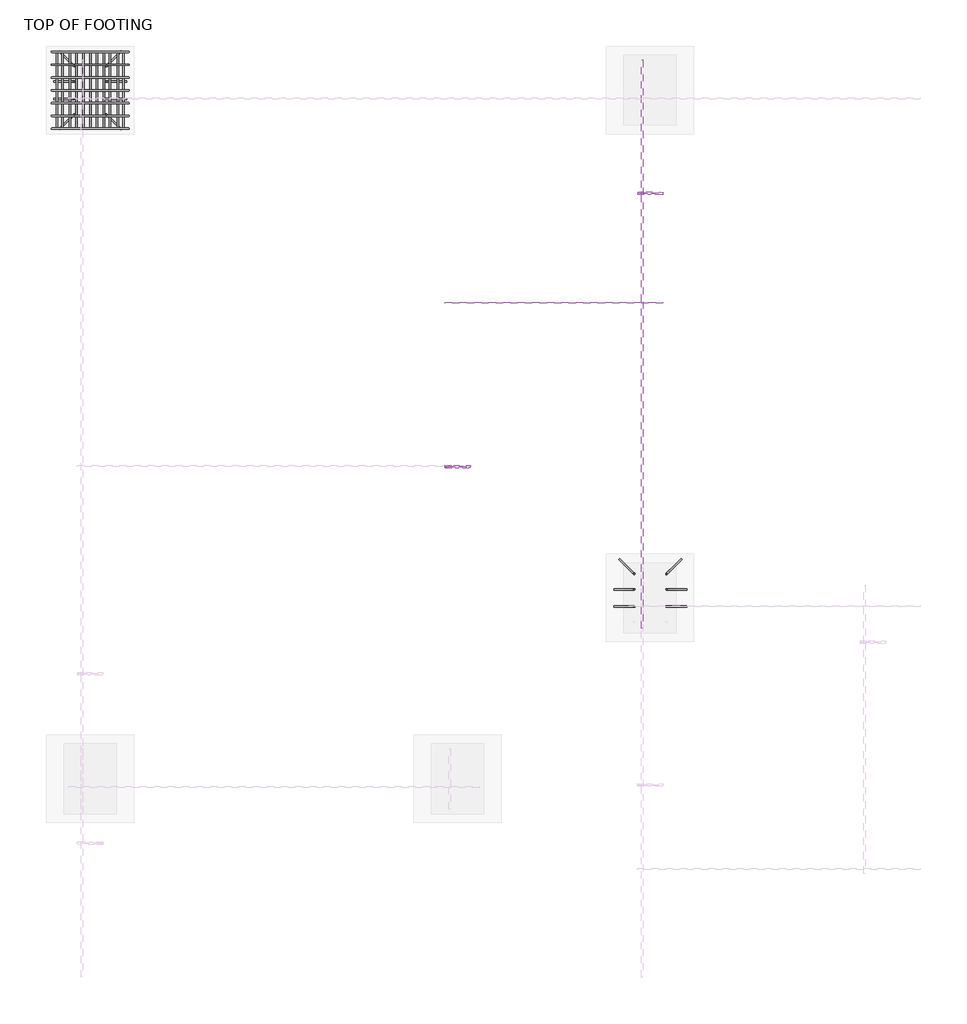
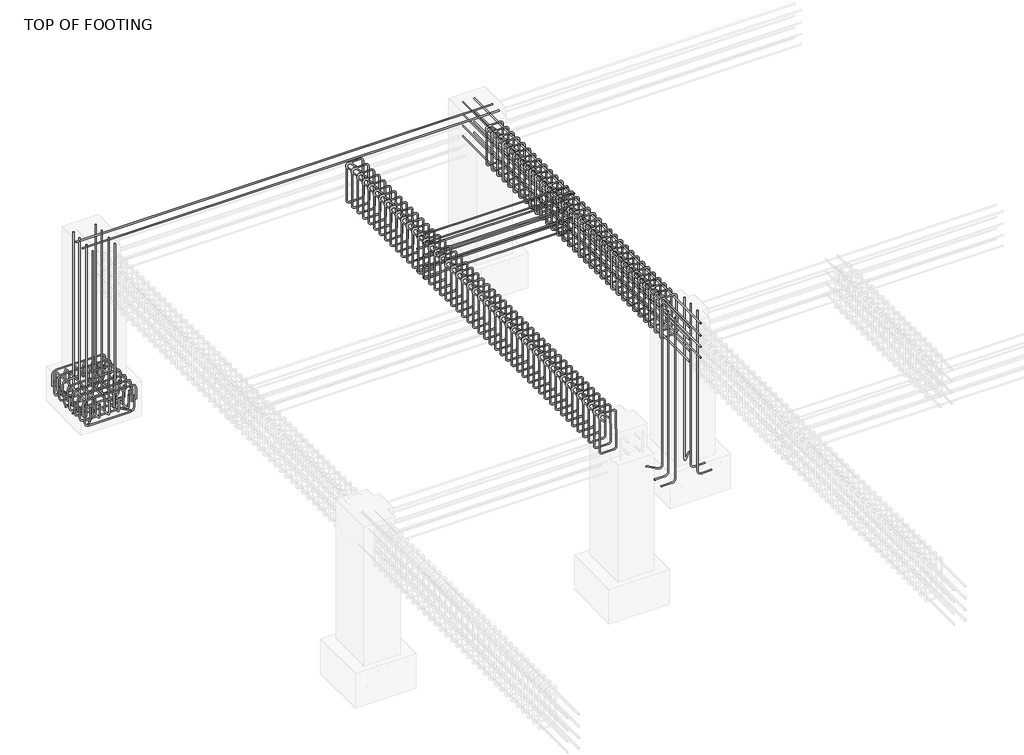
# One storey, part 6 of 8: 25 reinforcing bars.
"""IFC4 building model written with IfcOpenShell, lengths in millimetres."""

from ifc_helpers import new_model, si_unit, point, frame, origin, place, context, project, spatial, polyline, circle_curve, trimmed, segment, composite_curve, source, transform, mapped, element, save
from ifc_brep_helpers import swept_disk

model = new_model("IFC4")

# Units and contexts
model_context = context("Model", 3, world=origin())
ifc_project = project(units=[si_unit("LENGTHUNIT", "METRE", prefix="MILLI")], contexts=[model_context])

# Site, building, storey
site = spatial("IfcSite", under=ifc_project)
building = spatial("IfcBuilding", under=site)
storey = spatial("IfcBuildingStorey", under=building, Name="TOP OF FOOTING", Elevation=-1828.8)

# Reinforcing bars
placement = place(None, origin())
reinforcing_bar_shape = source(origin(), model_context, "Body", "SolidModel", [
    swept_disk(composite_curve([segment(polyline([(-6195.5877818, 9895.6420243, -2021.245224), (-6195.5877818, 9895.6420243, -2168.545224)]), True, "CONTINUOUS"), segment(trimmed(circle_curve(frame((-6241.9377818, 9895.6420243, -2168.545224), z_axis=(0.0, 1.0, 0.0), x_axis=(46.350000000000364, 0.0, 0.0)), 46.35), [point((-6195.5877818, 9895.6420243, -2168.545224))], [point((-6241.9377818, 9895.6420243, -2214.895224))], True, "CARTESIAN"), True, "CONTINUOUS"), segment(polyline([(-6241.9377818, 9895.6420243, -2214.895224), (-6762.8758647, 9895.6420243, -2214.895224)]), True, "CONTINUOUS"), segment(trimmed(circle_curve(frame((-6762.8758647, 9895.6420243, -2168.545224), z_axis=(0.0, 1.0, 0.0), x_axis=(0.0, 0.0, -46.34999999999991)), 46.35), [point((-6762.8758647, 9895.6420243, -2214.895224))], [point((-6809.2258647, 9895.6420243, -2168.545224))], True, "CARTESIAN"), True, "CONTINUOUS"), segment(polyline([(-6809.2258647, 9895.6420243, -2168.545224), (-6809.2258647, 9895.6420243, -2021.245224)]), True, "CONTINUOUS")], self_intersect=False), 6.35),
])
element("IfcReinforcingBar", 1, at=placement, inside=storey, context=model_context, shape_type="MappedRepresentation", body=[
    mapped(reinforcing_bar_shape, transform((0.0, 0.0, 0.0), x_axis=(1.0, 0.0, 0.0), y_axis=(0.0, 1.0, 0.0), z_axis=(0.0, 0.0, 1.0))),
    mapped(reinforcing_bar_shape, transform((0.0, -109.55, 0.0), x_axis=(1.0, 0.0, 0.0), y_axis=(0.0, 1.0, 0.0), z_axis=(0.0, 0.0, 1.0))),
    mapped(reinforcing_bar_shape, transform((0.0, -219.1, 0.0), x_axis=(1.0, 0.0, 0.0), y_axis=(0.0, 1.0, 0.0), z_axis=(0.0, 0.0, 1.0))),
    mapped(reinforcing_bar_shape, transform((0.0, -328.65, 0.0), x_axis=(1.0, 0.0, 0.0), y_axis=(0.0, 1.0, 0.0), z_axis=(0.0, 0.0, 1.0))),
    mapped(reinforcing_bar_shape, transform((0.0, -438.2, 0.0), x_axis=(1.0, 0.0, 0.0), y_axis=(0.0, 1.0, 0.0), z_axis=(0.0, 0.0, 1.0))),
    mapped(reinforcing_bar_shape, transform((0.0, -547.75, 0.0), x_axis=(1.0, 0.0, 0.0), y_axis=(0.0, 1.0, 0.0), z_axis=(0.0, 0.0, 1.0))),
    mapped(reinforcing_bar_shape, transform((0.0, -657.3, 0.0), x_axis=(1.0, 0.0, 0.0), y_axis=(0.0, 1.0, 0.0), z_axis=(0.0, 0.0, 1.0))),
])
reinforcing_bar_2_shape = source(origin(), model_context, "Body", "SolidModel", [
    swept_disk(composite_curve([segment(polyline([(-6831.1461367, 9895.6420243, -2068.8), (-6831.1461367, 9895.6420243, -1921.5)]), True, "CONTINUOUS"), segment(trimmed(circle_curve(frame((-6784.7961367, 9895.6420243, -1921.5), z_axis=(0.0, 1.0, 0.0), x_axis=(-46.350000000000364, 0.0, 0.0)), 46.35), [point((-6831.1461367, 9895.6420243, -1921.5))], [point((-6784.7961367, 9895.6420243, -1875.15))], True, "CARTESIAN"), True, "CONTINUOUS"), segment(polyline([(-6784.7961367, 9895.6420243, -1875.15), (-6220.1961367, 9895.6420243, -1875.15)]), True, "CONTINUOUS"), segment(trimmed(circle_curve(frame((-6220.1961367, 9895.6420243, -1921.5), z_axis=(0.0, 1.0, 0.0), x_axis=(0.0, 0.0, 46.34999999999991)), 46.35), [point((-6220.1961367, 9895.6420243, -1875.15))], [point((-6173.8461367, 9895.6420243, -1921.5))], True, "CARTESIAN"), True, "CONTINUOUS"), segment(polyline([(-6173.8461367, 9895.6420243, -1921.5), (-6173.8461367, 9895.6420243, -2068.8)]), True, "CONTINUOUS")], self_intersect=False), 6.35),
])
element("IfcReinforcingBar", 2, at=placement, inside=storey, context=model_context, shape_type="MappedRepresentation", body=[
    mapped(reinforcing_bar_2_shape, transform((0.0, 0.0, 0.0), x_axis=(1.0, 0.0, 0.0), y_axis=(0.0, 1.0, 0.0), z_axis=(0.0, 0.0, 1.0))),
    mapped(reinforcing_bar_2_shape, transform((0.0, -109.55, 0.0), x_axis=(1.0, 0.0, 0.0), y_axis=(0.0, 1.0, 0.0), z_axis=(0.0, 0.0, 1.0))),
    mapped(reinforcing_bar_2_shape, transform((0.0, -219.1, 0.0), x_axis=(1.0, 0.0, 0.0), y_axis=(0.0, 1.0, 0.0), z_axis=(0.0, 0.0, 1.0))),
    mapped(reinforcing_bar_2_shape, transform((0.0, -328.65, 0.0), x_axis=(1.0, 0.0, 0.0), y_axis=(0.0, 1.0, 0.0), z_axis=(0.0, 0.0, 1.0))),
    mapped(reinforcing_bar_2_shape, transform((0.0, -438.2, 0.0), x_axis=(1.0, 0.0, 0.0), y_axis=(0.0, 1.0, 0.0), z_axis=(0.0, 0.0, 1.0))),
    mapped(reinforcing_bar_2_shape, transform((0.0, -547.75, 0.0), x_axis=(1.0, 0.0, 0.0), y_axis=(0.0, 1.0, 0.0), z_axis=(0.0, 0.0, 1.0))),
    mapped(reinforcing_bar_2_shape, transform((0.0, -657.3, 0.0), x_axis=(1.0, 0.0, 0.0), y_axis=(0.0, 1.0, 0.0), z_axis=(0.0, 0.0, 1.0))),
])
reinforcing_bar_3_shape = source(origin(), model_context, "Body", "SolidModel", [
    swept_disk(composite_curve([segment(polyline([(-6219.0253093, 9895.6420243, -2080.9203068), (-6219.0253093, 9895.6420243, -1933.6203068)]), True, "CONTINUOUS"), segment(trimmed(circle_curve(frame((-6219.0253093, 9849.2920243, -1933.6203068), z_axis=(1.0, 0.0, 0.0), x_axis=(0.0, 46.349999999998545, 0.0)), 46.35), [point((-6219.0253093, 9895.6420243, -1933.6203068))], [point((-6219.0253093, 9849.2920243, -1887.2703068))], True, "CARTESIAN"), True, "CONTINUOUS"), segment(polyline([(-6219.0253093, 9849.2920243, -1887.2703068), (-6219.0253093, 9284.6920243, -1887.2703068)]), True, "CONTINUOUS"), segment(trimmed(circle_curve(frame((-6219.0253093, 9284.6920243, -1933.6203068), z_axis=(1.0, 0.0, 0.0), x_axis=(0.0, 0.0, 46.34999999999991)), 46.35), [point((-6219.0253093, 9284.6920243, -1887.2703068))], [point((-6219.0253093, 9238.3420243, -1933.6203068))], True, "CARTESIAN"), True, "CONTINUOUS"), segment(polyline([(-6219.0253093, 9238.3420243, -1933.6203068), (-6219.0253093, 9238.3420243, -2080.9203068)]), True, "CONTINUOUS")], self_intersect=False), 6.35),
])
element("IfcReinforcingBar", 3, at=placement, inside=storey, context=model_context, shape_type="MappedRepresentation", body=[
    mapped(reinforcing_bar_3_shape, transform((0.0, 0.0, 0.0), x_axis=(1.0, 0.0, 0.0), y_axis=(0.0, 1.0, 0.0), z_axis=(0.0, 0.0, 1.0))),
    mapped(reinforcing_bar_3_shape, transform((-113.9683653, 0.0, 0.0), x_axis=(1.0, 0.0, 0.0), y_axis=(0.0, 1.0, 0.0), z_axis=(0.0, 0.0, 1.0))),
    mapped(reinforcing_bar_3_shape, transform((-227.9367307, 0.0, 0.0), x_axis=(1.0, 0.0, 0.0), y_axis=(0.0, 1.0, 0.0), z_axis=(0.0, 0.0, 1.0))),
    mapped(reinforcing_bar_3_shape, transform((-341.905096, 0.0, 0.0), x_axis=(1.0, 0.0, 0.0), y_axis=(0.0, 1.0, 0.0), z_axis=(0.0, 0.0, 1.0))),
    mapped(reinforcing_bar_3_shape, transform((-455.8734613, 0.0, 0.0), x_axis=(1.0, 0.0, 0.0), y_axis=(0.0, 1.0, 0.0), z_axis=(0.0, 0.0, 1.0))),
    mapped(reinforcing_bar_3_shape, transform((-569.8418267, 0.0, 0.0), x_axis=(1.0, 0.0, 0.0), y_axis=(0.0, 1.0, 0.0), z_axis=(0.0, 0.0, 1.0))),
])
reinforcing_bar_4_shape = source(origin(), model_context, "Body", "SolidModel", [
    swept_disk(composite_curve([segment(polyline([(-6741.3656272, 9895.6420243, -1984.9681267), (-6741.3656272, 9895.6420243, -2132.2681267)]), True, "CONTINUOUS"), segment(trimmed(circle_curve(frame((-6741.3656272, 9849.2920243, -2132.2681267), z_axis=(-1.0, 0.0, 0.0), x_axis=(0.0, 46.349999999998545, 0.0)), 46.35), [point((-6741.3656272, 9895.6420243, -2132.2681267))], [point((-6741.3656272, 9849.2920243, -2178.6181267))], True, "CARTESIAN"), True, "CONTINUOUS"), segment(polyline([(-6741.3656272, 9849.2920243, -2178.6181267), (-6741.3656272, 9284.6920243, -2178.6181267)]), True, "CONTINUOUS"), segment(trimmed(circle_curve(frame((-6741.3656272, 9284.6920243, -2132.2681267), z_axis=(-1.0, 0.0, 0.0), x_axis=(0.0, 0.0, -46.350000000000364)), 46.35), [point((-6741.3656272, 9284.6920243, -2178.6181267))], [point((-6741.3656272, 9238.3420243, -2132.2681267))], True, "CARTESIAN"), True, "CONTINUOUS"), segment(polyline([(-6741.3656272, 9238.3420243, -2132.2681267), (-6741.3656272, 9238.3420243, -1984.9681267)]), True, "CONTINUOUS")], self_intersect=False), 6.35),
])
element("IfcReinforcingBar", 4, at=placement, inside=storey, context=model_context, shape_type="MappedRepresentation", body=[
    mapped(reinforcing_bar_4_shape, transform((0.0, 0.0, 0.0), x_axis=(1.0, 0.0, 0.0), y_axis=(0.0, 1.0, 0.0), z_axis=(0.0, 0.0, 1.0))),
    mapped(reinforcing_bar_4_shape, transform((119.2770606, 0.0, 0.0), x_axis=(1.0, 0.0, 0.0), y_axis=(0.0, 1.0, 0.0), z_axis=(0.0, 0.0, 1.0))),
    mapped(reinforcing_bar_4_shape, transform((238.5541211, 0.0, 0.0), x_axis=(1.0, 0.0, 0.0), y_axis=(0.0, 1.0, 0.0), z_axis=(0.0, 0.0, 1.0))),
    mapped(reinforcing_bar_4_shape, transform((357.8311817, 0.0, 0.0), x_axis=(1.0, 0.0, 0.0), y_axis=(0.0, 1.0, 0.0), z_axis=(0.0, 0.0, 1.0))),
    mapped(reinforcing_bar_4_shape, transform((477.1082423, 0.0, 0.0), x_axis=(1.0, 0.0, 0.0), y_axis=(0.0, 1.0, 0.0), z_axis=(0.0, 0.0, 1.0))),
])
reinforcing_bar_5_shape = source(origin(), model_context, "Body", "SolidModel", [
    swept_disk(composite_curve([segment(polyline([(-6815.4438347, 9642.1344308, -2192.6897268), (-6687.1151723, 9642.1344308, -2192.6897268)]), True, "CONTINUOUS"), segment(trimmed(circle_curve(frame((-6687.1151723, 9642.1344308, -2146.3397268), z_axis=(0.0, -1.0, 0.0), x_axis=(0.0, 0.0, -46.34999999999991)), 46.35), [point((-6687.1151723, 9642.1344308, -2192.6897268))], [point((-6640.7651723, 9642.1344308, -2146.3397268))], True, "CARTESIAN"), True, "CONTINUOUS"), segment(polyline([(-6640.7651723, 9642.1344308, -2146.3397268), (-6640.7651723, 9642.1344308, -40.0)]), True, "CONTINUOUS")], self_intersect=False), 6.35),
])
element("IfcReinforcingBar", 5, at=placement, inside=storey, context=model_context, shape_type="MappedRepresentation", body=[
    mapped(reinforcing_bar_5_shape, transform((0.0, 0.0, 0.0), x_axis=(1.0, 0.0, 0.0), y_axis=(0.0, 1.0, 0.0), z_axis=(0.0, 0.0, 1.0))),
    mapped(reinforcing_bar_5_shape, transform((0.0, -147.7903727, 0.0), x_axis=(1.0, 0.0, 0.0), y_axis=(0.0, 1.0, 0.0), z_axis=(0.0, 0.0, 1.0))),
])
element("IfcReinforcingBar", 6, at=placement, inside=storey, context=model_context, shape_type="SolidModel", body=[
    swept_disk(composite_curve([segment(polyline([(-6768.0144002, 9232.6300935, -2192.6897268), (-6673.5395717, 9327.1049221, -2192.6897268)]), True, "CONTINUOUS"), segment(trimmed(circle_curve(frame((-6673.5395717, 9327.1049221, -2146.3397268), z_axis=(0.7071067811865476, -0.7071067811865475, 0.0), x_axis=(0.0, 0.0, -46.34999999999991)), 46.35), [point((-6673.5395717, 9327.1049221, -2192.6897268))], [point((-6640.7651723, 9359.8793214, -2146.3397268))], True, "CARTESIAN"), True, "CONTINUOUS"), segment(polyline([(-6640.7651723, 9359.8793214, -2146.3397268), (-6640.7651723, 9359.8793214, -40.0)]), True, "CONTINUOUS")], self_intersect=False), 6.35),
])
element("IfcReinforcingBar", 7, at=placement, inside=storey, context=model_context, shape_type="SolidModel", body=[
    swept_disk(composite_curve([segment(polyline([(-6236.9778732, 9232.6300935, -2192.6897268), (-6331.4527018, 9327.1049221, -2192.6897268)]), True, "CONTINUOUS"), segment(trimmed(circle_curve(frame((-6331.4527018, 9327.1049221, -2146.3397268), z_axis=(0.7071067811865753, 0.7071067811865197, 0.0), x_axis=(0.0, 0.0, -46.34999999999991)), 46.35), [point((-6331.4527018, 9327.1049221, -2192.6897268))], [point((-6364.2271011, 9359.8793214, -2146.3397268))], True, "CARTESIAN"), True, "CONTINUOUS"), segment(polyline([(-6364.2271011, 9359.8793214, -2146.3397268), (-6364.2271011, 9359.8793214, -40.0)]), True, "CONTINUOUS")], self_intersect=False), 6.35),
])
element("IfcReinforcingBar", 8, at=placement, inside=storey, context=model_context, shape_type="SolidModel", body=[
    swept_disk(composite_curve([segment(polyline([(-6768.0144002, 9901.353955, -2192.6897268), (-6673.5395717, 9806.8791264, -2192.6897268)]), True, "CONTINUOUS"), segment(trimmed(circle_curve(frame((-6673.5395717, 9806.8791264, -2146.3397268), z_axis=(-0.7071067811865389, -0.7071067811865561, 0.0), x_axis=(0.0, 0.0, -46.34999999999991)), 46.35), [point((-6673.5395717, 9806.8791264, -2192.6897268))], [point((-6640.7651723, 9774.1047271, -2146.3397268))], True, "CARTESIAN"), True, "CONTINUOUS"), segment(polyline([(-6640.7651723, 9774.1047271, -2146.3397268), (-6640.7651723, 9774.1047271, -40.0)]), True, "CONTINUOUS")], self_intersect=False), 6.35),
])
element("IfcReinforcingBar", 9, at=placement, inside=storey, context=model_context, shape_type="SolidModel", body=[
    swept_disk(composite_curve([segment(polyline([(-6236.9778732, 9901.353955, -2192.6897268), (-6331.4527018, 9806.8791264, -2192.6897268)]), True, "CONTINUOUS"), segment(trimmed(circle_curve(frame((-6331.4527018, 9806.8791264, -2146.3397268), z_axis=(-0.707106781186584, 0.707106781186511, 0.0), x_axis=(0.0, 0.0, -46.34999999999991)), 46.35), [point((-6331.4527018, 9806.8791264, -2192.6897268))], [point((-6364.2271011, 9774.1047271, -2146.3397268))], True, "CARTESIAN"), True, "CONTINUOUS"), segment(polyline([(-6364.2271011, 9774.1047271, -2146.3397268), (-6364.2271011, 9774.1047271, -40.0)]), True, "CONTINUOUS")], self_intersect=False), 6.35),
])
reinforcing_bar_6_shape = source(origin(), model_context, "Body", "SolidModel", [
    swept_disk(composite_curve([segment(polyline([(-6189.5484388, 9642.1344308, -2192.6897268), (-6317.8771011, 9642.1344308, -2192.6897268)]), True, "CONTINUOUS"), segment(trimmed(circle_curve(frame((-6317.8771011, 9642.1344308, -2146.3397268), z_axis=(0.0, 1.0, 0.0), x_axis=(0.0, 0.0, -46.34999999999991)), 46.35), [point((-6317.8771011, 9642.1344308, -2192.6897268))], [point((-6364.2271011, 9642.1344308, -2146.3397268))], True, "CARTESIAN"), True, "CONTINUOUS"), segment(polyline([(-6364.2271011, 9642.1344308, -2146.3397268), (-6364.2271011, 9642.1344308, -40.0)]), True, "CONTINUOUS")], self_intersect=False), 6.35),
])
element("IfcReinforcingBar", 10, at=placement, inside=storey, context=model_context, shape_type="MappedRepresentation", body=[
    mapped(reinforcing_bar_6_shape, transform((0.0, 0.0, 0.0), x_axis=(1.0, 0.0, 0.0), y_axis=(0.0, 1.0, 0.0), z_axis=(0.0, 0.0, 1.0))),
    mapped(reinforcing_bar_6_shape, transform((0.0, -147.7903727, 0.0), x_axis=(1.0, 0.0, 0.0), y_axis=(0.0, 1.0, 0.0), z_axis=(0.0, 0.0, 1.0))),
])
reinforcing_bar_7_shape = source(origin(), model_context, "Body", "SolidModel", [
    swept_disk(composite_curve([segment(polyline([(-2015.4438347, 5292.1344308, -2192.6897268), (-1887.1151723, 5292.1344308, -2192.6897268)]), True, "CONTINUOUS"), segment(trimmed(circle_curve(frame((-1887.1151723, 5292.1344308, -2146.3397268), z_axis=(0.0, -1.0, 0.0), x_axis=(0.0, 0.0, -46.34999999999991)), 46.35), [point((-1887.1151723, 5292.1344308, -2192.6897268))], [point((-1840.7651723, 5292.1344308, -2146.3397268))], True, "CARTESIAN"), True, "CONTINUOUS"), segment(polyline([(-1840.7651723, 5292.1344308, -2146.3397268), (-1840.7651723, 5292.1344308, -40.0)]), True, "CONTINUOUS")], self_intersect=False), 6.35),
])
element("IfcReinforcingBar", 11, at=placement, inside=storey, context=model_context, shape_type="MappedRepresentation", body=[
    mapped(reinforcing_bar_7_shape, transform((0.0, 0.0, 0.0), x_axis=(1.0, 0.0, 0.0), y_axis=(0.0, 1.0, 0.0), z_axis=(0.0, 0.0, 1.0))),
    mapped(reinforcing_bar_7_shape, transform((0.0, -147.7903727, 0.0), x_axis=(1.0, 0.0, 0.0), y_axis=(0.0, 1.0, 0.0), z_axis=(0.0, 0.0, 1.0))),
])
element("IfcReinforcingBar", 12, at=placement, inside=storey, context=model_context, shape_type="SolidModel", body=[
    swept_disk(composite_curve([segment(polyline([(-1968.0144002, 5551.353955, -2192.6897268), (-1873.5395717, 5456.8791264, -2192.6897268)]), True, "CONTINUOUS"), segment(trimmed(circle_curve(frame((-1873.5395717, 5456.8791264, -2146.3397268), z_axis=(-0.7071067811865389, -0.7071067811865561, 0.0), x_axis=(0.0, 0.0, -46.34999999999991)), 46.35), [point((-1873.5395717, 5456.8791264, -2192.6897268))], [point((-1840.7651723, 5424.1047271, -2146.3397268))], True, "CARTESIAN"), True, "CONTINUOUS"), segment(polyline([(-1840.7651723, 5424.1047271, -2146.3397268), (-1840.7651723, 5424.1047271, -40.0)]), True, "CONTINUOUS")], self_intersect=False), 6.35),
])
element("IfcReinforcingBar", 13, at=placement, inside=storey, context=model_context, shape_type="SolidModel", body=[
    swept_disk(composite_curve([segment(polyline([(-1436.9778732, 5551.353955, -2192.6897268), (-1531.4527018, 5456.8791264, -2192.6897268)]), True, "CONTINUOUS"), segment(trimmed(circle_curve(frame((-1531.4527018, 5456.8791264, -2146.3397268), z_axis=(-0.707106781186584, 0.707106781186511, 0.0), x_axis=(0.0, 0.0, -46.34999999999991)), 46.35), [point((-1531.4527018, 5456.8791264, -2192.6897268))], [point((-1564.2271011, 5424.1047271, -2146.3397268))], True, "CARTESIAN"), True, "CONTINUOUS"), segment(polyline([(-1564.2271011, 5424.1047271, -2146.3397268), (-1564.2271011, 5424.1047271, -40.0)]), True, "CONTINUOUS")], self_intersect=False), 6.35),
])
reinforcing_bar_8_shape = source(origin(), model_context, "Body", "SolidModel", [
    swept_disk(composite_curve([segment(polyline([(-1389.5484388, 5292.1344308, -2192.6897268), (-1517.8771011, 5292.1344308, -2192.6897268)]), True, "CONTINUOUS"), segment(trimmed(circle_curve(frame((-1517.8771011, 5292.1344308, -2146.3397268), z_axis=(0.0, 1.0, 0.0), x_axis=(0.0, 0.0, -46.34999999999991)), 46.35), [point((-1517.8771011, 5292.1344308, -2192.6897268))], [point((-1564.2271011, 5292.1344308, -2146.3397268))], True, "CARTESIAN"), True, "CONTINUOUS"), segment(polyline([(-1564.2271011, 5292.1344308, -2146.3397268), (-1564.2271011, 5292.1344308, -40.0)]), True, "CONTINUOUS")], self_intersect=False), 6.35),
])
element("IfcReinforcingBar", 14, at=placement, inside=storey, context=model_context, shape_type="MappedRepresentation", body=[
    mapped(reinforcing_bar_8_shape, transform((0.0, 0.0, 0.0), x_axis=(1.0, 0.0, 0.0), y_axis=(0.0, 1.0, 0.0), z_axis=(0.0, 0.0, 1.0))),
    mapped(reinforcing_bar_8_shape, transform((0.0, -147.7903727, 0.0), x_axis=(1.0, 0.0, 0.0), y_axis=(0.0, 1.0, 0.0), z_axis=(0.0, 0.0, 1.0))),
])
reinforcing_bar_9_shape = source(origin(), model_context, "Body", "SolidModel", [
    swept_disk(composite_curve([segment(polyline([(-6687.4961367, 9636.6137956, -72.7), (-1517.4961367, 9636.6137956, -72.7)]), True, "CONTINUOUS")], self_intersect=False), 6.35),
])
element("IfcReinforcingBar", 15, at=placement, inside=storey, context=model_context, shape_type="MappedRepresentation", body=[
    mapped(reinforcing_bar_9_shape, transform((0.0, 0.0, 0.0), x_axis=(1.0, 0.0, 0.0), y_axis=(0.0, 1.0, 0.0), z_axis=(0.0, 0.0, 1.0))),
    mapped(reinforcing_bar_9_shape, transform((0.0, -139.7429418, 0.0), x_axis=(1.0, 0.0, 0.0), y_axis=(0.0, 1.0, 0.0), z_axis=(0.0, 0.0, 1.0))),
])
reinforcing_bar_10_shape = source(origin(), model_context, "Body", "SolidModel", [
    swept_disk(composite_curve([segment(polyline([(-1696.8847762, 9260.6420243, -111.2757654), (-1752.6283391, 9260.6420243, -55.5322024)]), True, "CONTINUOUS"), segment(trimmed(circle_curve(frame((-1774.7961367, 9260.6420243, -77.7), z_axis=(0.0, -1.0, 0.0), x_axis=(22.167797600000085, 0.0, 22.1677976)), 31.35), [point((-1752.6283391, 9260.6420243, -55.5322024))], [point((-1806.1461367, 9260.6420243, -77.7))], True, "CARTESIAN"), True, "CONTINUOUS"), segment(polyline([(-1806.1461367, 9260.6420243, -77.7), (-1806.1461367, 9260.6420243, -522.3)]), True, "CONTINUOUS"), segment(trimmed(circle_curve(frame((-1774.7961367, 9260.6420243, -522.3), z_axis=(0.0, -1.0, 0.0), x_axis=(-31.34999999999991, 0.0, 0.0)), 31.35), [point((-1806.1461367, 9260.6420243, -522.3))], [point((-1774.7961367, 9260.6420243, -553.65))], True, "CARTESIAN"), True, "CONTINUOUS"), segment(polyline([(-1774.7961367, 9260.6420243, -553.65), (-1630.1961367, 9260.6420243, -553.65)]), True, "CONTINUOUS"), segment(trimmed(circle_curve(frame((-1630.1961367, 9261.4266099, -522.3098193), z_axis=(0.0, -0.9996867842138424, 0.025026655153786322), x_axis=(0.0, -0.784585600000355, -31.34018070000002)), 31.35), [point((-1630.1961367, 9260.6420243, -553.65))], [point((-1598.8461367, 9261.4266099, -522.3098193))], True, "CARTESIAN"), True, "CONTINUOUS"), segment(polyline([(-1598.8461367, 9261.4266099, -522.3098193), (-1598.8461367, 9272.5574386, -77.6901807)]), True, "CONTINUOUS"), segment(trimmed(circle_curve(frame((-1630.1961367, 9272.5574386, -77.6901807), z_axis=(0.0, -0.9996867842138424, 0.025026655153786322), x_axis=(31.34999999999991, 0.0, 0.0)), 31.35), [point((-1598.8461367, 9272.5574386, -77.6901807))], [point((-1630.1961367, 9273.3420243, -46.35))], True, "CARTESIAN"), True, "CONTINUOUS"), segment(polyline([(-1630.1961367, 9273.3420243, -46.35), (-1774.7961367, 9273.3420243, -46.35)]), True, "CONTINUOUS"), segment(trimmed(circle_curve(frame((-1774.7961367, 9273.3420243, -77.7), z_axis=(0.0, -1.0, 0.0), x_axis=(0.0, 0.0, 31.35)), 31.35), [point((-1774.7961367, 9273.3420243, -46.35))], [point((-1796.9639343, 9273.3420243, -99.8677976))], True, "CARTESIAN"), True, "CONTINUOUS"), segment(polyline([(-1796.9639343, 9273.3420243, -99.8677976), (-1741.2203714, 9273.3420243, -155.6113605)]), True, "CONTINUOUS")], self_intersect=False), 6.35),
])
element("IfcReinforcingBar", 16, at=placement, inside=storey, context=model_context, shape_type="MappedRepresentation", body=[
    mapped(reinforcing_bar_10_shape, transform((0.0, 0.0, 0.0), x_axis=(1.0, 0.0, 0.0), y_axis=(0.0, 1.0, 0.0), z_axis=(0.0, 0.0, 1.0))),
    mapped(reinforcing_bar_10_shape, transform((0.0, -116.790625, 0.0), x_axis=(1.0, 0.0, 0.0), y_axis=(0.0, 1.0, 0.0), z_axis=(0.0, 0.0, 1.0))),
    mapped(reinforcing_bar_10_shape, transform((0.0, -233.58125, 0.0), x_axis=(1.0, 0.0, 0.0), y_axis=(0.0, 1.0, 0.0), z_axis=(0.0, 0.0, 1.0))),
    mapped(reinforcing_bar_10_shape, transform((0.0, -350.371875, 0.0), x_axis=(1.0, 0.0, 0.0), y_axis=(0.0, 1.0, 0.0), z_axis=(0.0, 0.0, 1.0))),
    mapped(reinforcing_bar_10_shape, transform((0.0, -467.1625, 0.0), x_axis=(1.0, 0.0, 0.0), y_axis=(0.0, 1.0, 0.0), z_axis=(0.0, 0.0, 1.0))),
    mapped(reinforcing_bar_10_shape, transform((0.0, -583.953125, 0.0), x_axis=(1.0, 0.0, 0.0), y_axis=(0.0, 1.0, 0.0), z_axis=(0.0, 0.0, 1.0))),
    mapped(reinforcing_bar_10_shape, transform((0.0, -700.74375, 0.0), x_axis=(1.0, 0.0, 0.0), y_axis=(0.0, 1.0, 0.0), z_axis=(0.0, 0.0, 1.0))),
    mapped(reinforcing_bar_10_shape, transform((0.0, -817.534375, 0.0), x_axis=(1.0, 0.0, 0.0), y_axis=(0.0, 1.0, 0.0), z_axis=(0.0, 0.0, 1.0))),
    mapped(reinforcing_bar_10_shape, transform((0.0, -934.325, 0.0), x_axis=(1.0, 0.0, 0.0), y_axis=(0.0, 1.0, 0.0), z_axis=(0.0, 0.0, 1.0))),
    mapped(reinforcing_bar_10_shape, transform((0.0, -1051.115625, 0.0), x_axis=(1.0, 0.0, 0.0), y_axis=(0.0, 1.0, 0.0), z_axis=(0.0, 0.0, 1.0))),
    mapped(reinforcing_bar_10_shape, transform((0.0, -1167.90625, 0.0), x_axis=(1.0, 0.0, 0.0), y_axis=(0.0, 1.0, 0.0), z_axis=(0.0, 0.0, 1.0))),
    mapped(reinforcing_bar_10_shape, transform((0.0, -1284.696875, 0.0), x_axis=(1.0, 0.0, 0.0), y_axis=(0.0, 1.0, 0.0), z_axis=(0.0, 0.0, 1.0))),
    mapped(reinforcing_bar_10_shape, transform((0.0, -1401.4875, 0.0), x_axis=(1.0, 0.0, 0.0), y_axis=(0.0, 1.0, 0.0), z_axis=(0.0, 0.0, 1.0))),
    mapped(reinforcing_bar_10_shape, transform((0.0, -1518.278125, 0.0), x_axis=(1.0, 0.0, 0.0), y_axis=(0.0, 1.0, 0.0), z_axis=(0.0, 0.0, 1.0))),
    mapped(reinforcing_bar_10_shape, transform((0.0, -1635.06875, 0.0), x_axis=(1.0, 0.0, 0.0), y_axis=(0.0, 1.0, 0.0), z_axis=(0.0, 0.0, 1.0))),
    mapped(reinforcing_bar_10_shape, transform((0.0, -1751.859375, 0.0), x_axis=(1.0, 0.0, 0.0), y_axis=(0.0, 1.0, 0.0), z_axis=(0.0, 0.0, 1.0))),
    mapped(reinforcing_bar_10_shape, transform((0.0, -1868.65, 0.0), x_axis=(1.0, 0.0, 0.0), y_axis=(0.0, 1.0, 0.0), z_axis=(0.0, 0.0, 1.0))),
    mapped(reinforcing_bar_10_shape, transform((0.0, -1985.440625, 0.0), x_axis=(1.0, 0.0, 0.0), y_axis=(0.0, 1.0, 0.0), z_axis=(0.0, 0.0, 1.0))),
    mapped(reinforcing_bar_10_shape, transform((0.0, -2102.23125, 0.0), x_axis=(1.0, 0.0, 0.0), y_axis=(0.0, 1.0, 0.0), z_axis=(0.0, 0.0, 1.0))),
    mapped(reinforcing_bar_10_shape, transform((0.0, -2219.021875, 0.0), x_axis=(1.0, 0.0, 0.0), y_axis=(0.0, 1.0, 0.0), z_axis=(0.0, 0.0, 1.0))),
    mapped(reinforcing_bar_10_shape, transform((0.0, -2335.8125, 0.0), x_axis=(1.0, 0.0, 0.0), y_axis=(0.0, 1.0, 0.0), z_axis=(0.0, 0.0, 1.0))),
    mapped(reinforcing_bar_10_shape, transform((0.0, -2452.603125, 0.0), x_axis=(1.0, 0.0, 0.0), y_axis=(0.0, 1.0, 0.0), z_axis=(0.0, 0.0, 1.0))),
    mapped(reinforcing_bar_10_shape, transform((0.0, -2569.39375, 0.0), x_axis=(1.0, 0.0, 0.0), y_axis=(0.0, 1.0, 0.0), z_axis=(0.0, 0.0, 1.0))),
    mapped(reinforcing_bar_10_shape, transform((0.0, -2686.184375, 0.0), x_axis=(1.0, 0.0, 0.0), y_axis=(0.0, 1.0, 0.0), z_axis=(0.0, 0.0, 1.0))),
    mapped(reinforcing_bar_10_shape, transform((0.0, -2802.975, 0.0), x_axis=(1.0, 0.0, 0.0), y_axis=(0.0, 1.0, 0.0), z_axis=(0.0, 0.0, 1.0))),
    mapped(reinforcing_bar_10_shape, transform((0.0, -2919.765625, 0.0), x_axis=(1.0, 0.0, 0.0), y_axis=(0.0, 1.0, 0.0), z_axis=(0.0, 0.0, 1.0))),
    mapped(reinforcing_bar_10_shape, transform((0.0, -3036.55625, 0.0), x_axis=(1.0, 0.0, 0.0), y_axis=(0.0, 1.0, 0.0), z_axis=(0.0, 0.0, 1.0))),
    mapped(reinforcing_bar_10_shape, transform((0.0, -3153.346875, 0.0), x_axis=(1.0, 0.0, 0.0), y_axis=(0.0, 1.0, 0.0), z_axis=(0.0, 0.0, 1.0))),
    mapped(reinforcing_bar_10_shape, transform((0.0, -3270.1375, 0.0), x_axis=(1.0, 0.0, 0.0), y_axis=(0.0, 1.0, 0.0), z_axis=(0.0, 0.0, 1.0))),
    mapped(reinforcing_bar_10_shape, transform((0.0, -3386.928125, 0.0), x_axis=(1.0, 0.0, 0.0), y_axis=(0.0, 1.0, 0.0), z_axis=(0.0, 0.0, 1.0))),
    mapped(reinforcing_bar_10_shape, transform((0.0, -3503.71875, 0.0), x_axis=(1.0, 0.0, 0.0), y_axis=(0.0, 1.0, 0.0), z_axis=(0.0, 0.0, 1.0))),
    mapped(reinforcing_bar_10_shape, transform((0.0, -3620.509375, 0.0), x_axis=(1.0, 0.0, 0.0), y_axis=(0.0, 1.0, 0.0), z_axis=(0.0, 0.0, 1.0))),
    mapped(reinforcing_bar_10_shape, transform((0.0, -3737.3, 0.0), x_axis=(1.0, 0.0, 0.0), y_axis=(0.0, 1.0, 0.0), z_axis=(0.0, 0.0, 1.0))),
])
reinforcing_bar_11_shape = source(origin(), model_context, "Body", "SolidModel", [
    swept_disk(composite_curve([segment(polyline([(-1632.8743653, 9826.9920243, -72.7), (-1632.8743653, 4956.9920243, -72.7)]), True, "CONTINUOUS")], self_intersect=False), 6.35),
])
element("IfcReinforcingBar", 17, at=placement, inside=storey, context=model_context, shape_type="MappedRepresentation", body=[
    mapped(reinforcing_bar_11_shape, transform((0.0, 0.0, 0.0), x_axis=(1.0, 0.0, 0.0), y_axis=(0.0, 1.0, 0.0), z_axis=(0.0, 0.0, 1.0))),
    mapped(reinforcing_bar_11_shape, transform((-139.7429418, 0.0, 0.0), x_axis=(1.0, 0.0, 0.0), y_axis=(0.0, 1.0, 0.0), z_axis=(0.0, 0.0, 1.0))),
])
reinforcing_bar_12_shape = source(origin(), model_context, "Body", "SolidModel", [
    swept_disk(composite_curve([segment(polyline([(-1632.8743653, 9826.9920243, -522.7), (-1632.8743653, 4956.9920243, -522.7)]), True, "CONTINUOUS")], self_intersect=False), 6.35),
])
element("IfcReinforcingBar", 18, at=placement, inside=storey, context=model_context, shape_type="MappedRepresentation", body=[
    mapped(reinforcing_bar_12_shape, transform((0.0, 0.0, 0.0), x_axis=(1.0, 0.0, 0.0), y_axis=(0.0, 1.0, 0.0), z_axis=(0.0, 0.0, 1.0))),
    mapped(reinforcing_bar_12_shape, transform((-139.7429418, 0.0, 0.0), x_axis=(1.0, 0.0, 0.0), y_axis=(0.0, 1.0, 0.0), z_axis=(0.0, 0.0, 1.0))),
])
reinforcing_bar_13_shape = source(origin(), model_context, "Body", "SolidModel", [
    swept_disk(composite_curve([segment(polyline([(-1632.8743653, 9826.9920243, -382.7), (-1632.8743653, 4956.9920243, -382.7)]), True, "CONTINUOUS")], self_intersect=False), 6.35),
])
element("IfcReinforcingBar", 19, at=placement, inside=storey, context=model_context, shape_type="MappedRepresentation", body=[
    mapped(reinforcing_bar_13_shape, transform((0.0, 0.0, 0.0), x_axis=(1.0, 0.0, 0.0), y_axis=(0.0, 1.0, 0.0), z_axis=(0.0, 0.0, 1.0))),
    mapped(reinforcing_bar_13_shape, transform((-139.7429418, 0.0, 0.0), x_axis=(1.0, 0.0, 0.0), y_axis=(0.0, 1.0, 0.0), z_axis=(0.0, 0.0, 1.0))),
])
reinforcing_bar_14_shape = source(origin(), model_context, "Body", "SolidModel", [
    swept_disk(composite_curve([segment(polyline([(-1632.8743653, 9826.9920243, -232.7), (-1632.8743653, 4956.9920243, -232.7)]), True, "CONTINUOUS")], self_intersect=False), 6.35),
])
element("IfcReinforcingBar", 20, at=placement, inside=storey, context=model_context, shape_type="MappedRepresentation", body=[
    mapped(reinforcing_bar_14_shape, transform((0.0, 0.0, 0.0), x_axis=(1.0, 0.0, 0.0), y_axis=(0.0, 1.0, 0.0), z_axis=(0.0, 0.0, 1.0))),
    mapped(reinforcing_bar_14_shape, transform((-139.7429418, 0.0, 0.0), x_axis=(1.0, 0.0, 0.0), y_axis=(0.0, 1.0, 0.0), z_axis=(0.0, 0.0, 1.0))),
])
reinforcing_bar_15_shape = source(origin(), model_context, "Body", "SolidModel", [
    swept_disk(composite_curve([segment(polyline([(-3346.8847762, 9410.6420243, -111.2757654), (-3402.6283391, 9410.6420243, -55.5322024)]), True, "CONTINUOUS"), segment(trimmed(circle_curve(frame((-3424.7961367, 9410.6420243, -77.7), z_axis=(0.0, -1.0, 0.0), x_axis=(22.16779759999963, 0.0, 22.1677976)), 31.35), [point((-3402.6283391, 9410.6420243, -55.5322024))], [point((-3456.1461367, 9410.6420243, -77.7))], True, "CARTESIAN"), True, "CONTINUOUS"), segment(polyline([(-3456.1461367, 9410.6420243, -77.7), (-3456.1461367, 9410.6420243, -522.3)]), True, "CONTINUOUS"), segment(trimmed(circle_curve(frame((-3424.7961367, 9410.6420243, -522.3), z_axis=(0.0, -1.0, 0.0), x_axis=(-31.350000000000364, 0.0, 0.0)), 31.35), [point((-3456.1461367, 9410.6420243, -522.3))], [point((-3424.7961367, 9410.6420243, -553.65))], True, "CARTESIAN"), True, "CONTINUOUS"), segment(polyline([(-3424.7961367, 9410.6420243, -553.65), (-3280.1961367, 9410.6420243, -553.65)]), True, "CONTINUOUS"), segment(trimmed(circle_curve(frame((-3280.1961367, 9411.4266099, -522.3098193), z_axis=(0.0, -0.9996867842138424, 0.025026655153786322), x_axis=(0.0, -0.784585600000355, -31.34018070000002)), 31.35), [point((-3280.1961367, 9410.6420243, -553.65))], [point((-3248.8461367, 9411.4266099, -522.3098193))], True, "CARTESIAN"), True, "CONTINUOUS"), segment(polyline([(-3248.8461367, 9411.4266099, -522.3098193), (-3248.8461367, 9422.5574386, -77.6901807)]), True, "CONTINUOUS"), segment(trimmed(circle_curve(frame((-3280.1961367, 9422.5574386, -77.6901807), z_axis=(0.0, -0.9996867842138424, 0.025026655153786322), x_axis=(31.34999999999991, 0.0, 0.0)), 31.35), [point((-3248.8461367, 9422.5574386, -77.6901807))], [point((-3280.1961367, 9423.3420243, -46.35))], True, "CARTESIAN"), True, "CONTINUOUS"), segment(polyline([(-3280.1961367, 9423.3420243, -46.35), (-3424.7961367, 9423.3420243, -46.35)]), True, "CONTINUOUS"), segment(trimmed(circle_curve(frame((-3424.7961367, 9423.3420243, -77.7), z_axis=(0.0, -1.0, 0.0), x_axis=(0.0, 0.0, 31.35)), 31.35), [point((-3424.7961367, 9423.3420243, -46.35))], [point((-3446.9639343, 9423.3420243, -99.8677976))], True, "CARTESIAN"), True, "CONTINUOUS"), segment(polyline([(-3446.9639343, 9423.3420243, -99.8677976), (-3391.2203714, 9423.3420243, -155.6113605)]), True, "CONTINUOUS")], self_intersect=False), 6.35),
])
element("IfcReinforcingBar", 21, at=placement, inside=storey, context=model_context, shape_type="MappedRepresentation", body=[
    mapped(reinforcing_bar_15_shape, transform((0.0, 0.0, 0.0), x_axis=(1.0, 0.0, 0.0), y_axis=(0.0, 1.0, 0.0), z_axis=(0.0, 0.0, 1.0))),
    mapped(reinforcing_bar_15_shape, transform((0.0, -118.2021739, 0.0), x_axis=(1.0, 0.0, 0.0), y_axis=(0.0, 1.0, 0.0), z_axis=(0.0, 0.0, 1.0))),
    mapped(reinforcing_bar_15_shape, transform((0.0, -236.4043478, 0.0), x_axis=(1.0, 0.0, 0.0), y_axis=(0.0, 1.0, 0.0), z_axis=(0.0, 0.0, 1.0))),
    mapped(reinforcing_bar_15_shape, transform((0.0, -354.6065217, 0.0), x_axis=(1.0, 0.0, 0.0), y_axis=(0.0, 1.0, 0.0), z_axis=(0.0, 0.0, 1.0))),
    mapped(reinforcing_bar_15_shape, transform((0.0, -472.8086957, 0.0), x_axis=(1.0, 0.0, 0.0), y_axis=(0.0, 1.0, 0.0), z_axis=(0.0, 0.0, 1.0))),
    mapped(reinforcing_bar_15_shape, transform((0.0, -591.0108696, 0.0), x_axis=(1.0, 0.0, 0.0), y_axis=(0.0, 1.0, 0.0), z_axis=(0.0, 0.0, 1.0))),
    mapped(reinforcing_bar_15_shape, transform((0.0, -709.2130435, 0.0), x_axis=(1.0, 0.0, 0.0), y_axis=(0.0, 1.0, 0.0), z_axis=(0.0, 0.0, 1.0))),
    mapped(reinforcing_bar_15_shape, transform((0.0, -827.4152174, 0.0), x_axis=(1.0, 0.0, 0.0), y_axis=(0.0, 1.0, 0.0), z_axis=(0.0, 0.0, 1.0))),
    mapped(reinforcing_bar_15_shape, transform((0.0, -945.6173913, 0.0), x_axis=(1.0, 0.0, 0.0), y_axis=(0.0, 1.0, 0.0), z_axis=(0.0, 0.0, 1.0))),
    mapped(reinforcing_bar_15_shape, transform((0.0, -1063.8195652, 0.0), x_axis=(1.0, 0.0, 0.0), y_axis=(0.0, 1.0, 0.0), z_axis=(0.0, 0.0, 1.0))),
    mapped(reinforcing_bar_15_shape, transform((0.0, -1182.0217391, 0.0), x_axis=(1.0, 0.0, 0.0), y_axis=(0.0, 1.0, 0.0), z_axis=(0.0, 0.0, 1.0))),
    mapped(reinforcing_bar_15_shape, transform((0.0, -1300.223913, 0.0), x_axis=(1.0, 0.0, 0.0), y_axis=(0.0, 1.0, 0.0), z_axis=(0.0, 0.0, 1.0))),
    mapped(reinforcing_bar_15_shape, transform((0.0, -1418.426087, 0.0), x_axis=(1.0, 0.0, 0.0), y_axis=(0.0, 1.0, 0.0), z_axis=(0.0, 0.0, 1.0))),
    mapped(reinforcing_bar_15_shape, transform((0.0, -1536.6282609, 0.0), x_axis=(1.0, 0.0, 0.0), y_axis=(0.0, 1.0, 0.0), z_axis=(0.0, 0.0, 1.0))),
    mapped(reinforcing_bar_15_shape, transform((0.0, -1654.8304348, 0.0), x_axis=(1.0, 0.0, 0.0), y_axis=(0.0, 1.0, 0.0), z_axis=(0.0, 0.0, 1.0))),
    mapped(reinforcing_bar_15_shape, transform((0.0, -1773.0326087, 0.0), x_axis=(1.0, 0.0, 0.0), y_axis=(0.0, 1.0, 0.0), z_axis=(0.0, 0.0, 1.0))),
    mapped(reinforcing_bar_15_shape, transform((0.0, -1891.2347826, 0.0), x_axis=(1.0, 0.0, 0.0), y_axis=(0.0, 1.0, 0.0), z_axis=(0.0, 0.0, 1.0))),
    mapped(reinforcing_bar_15_shape, transform((0.0, -2009.4369565, 0.0), x_axis=(1.0, 0.0, 0.0), y_axis=(0.0, 1.0, 0.0), z_axis=(0.0, 0.0, 1.0))),
    mapped(reinforcing_bar_15_shape, transform((0.0, -2127.6391304, 0.0), x_axis=(1.0, 0.0, 0.0), y_axis=(0.0, 1.0, 0.0), z_axis=(0.0, 0.0, 1.0))),
    mapped(reinforcing_bar_15_shape, transform((0.0, -2245.8413043, 0.0), x_axis=(1.0, 0.0, 0.0), y_axis=(0.0, 1.0, 0.0), z_axis=(0.0, 0.0, 1.0))),
    mapped(reinforcing_bar_15_shape, transform((0.0, -2364.0434783, 0.0), x_axis=(1.0, 0.0, 0.0), y_axis=(0.0, 1.0, 0.0), z_axis=(0.0, 0.0, 1.0))),
    mapped(reinforcing_bar_15_shape, transform((0.0, -2482.2456522, 0.0), x_axis=(1.0, 0.0, 0.0), y_axis=(0.0, 1.0, 0.0), z_axis=(0.0, 0.0, 1.0))),
    mapped(reinforcing_bar_15_shape, transform((0.0, -2600.4478261, 0.0), x_axis=(1.0, 0.0, 0.0), y_axis=(0.0, 1.0, 0.0), z_axis=(0.0, 0.0, 1.0))),
    mapped(reinforcing_bar_15_shape, transform((0.0, -2718.65, 0.0), x_axis=(1.0, 0.0, 0.0), y_axis=(0.0, 1.0, 0.0), z_axis=(0.0, 0.0, 1.0))),
    mapped(reinforcing_bar_15_shape, transform((0.0, -2836.8521739, 0.0), x_axis=(1.0, 0.0, 0.0), y_axis=(0.0, 1.0, 0.0), z_axis=(0.0, 0.0, 1.0))),
    mapped(reinforcing_bar_15_shape, transform((0.0, -2955.0543478, 0.0), x_axis=(1.0, 0.0, 0.0), y_axis=(0.0, 1.0, 0.0), z_axis=(0.0, 0.0, 1.0))),
    mapped(reinforcing_bar_15_shape, transform((0.0, -3073.2565217, 0.0), x_axis=(1.0, 0.0, 0.0), y_axis=(0.0, 1.0, 0.0), z_axis=(0.0, 0.0, 1.0))),
    mapped(reinforcing_bar_15_shape, transform((0.0, -3191.4586957, 0.0), x_axis=(1.0, 0.0, 0.0), y_axis=(0.0, 1.0, 0.0), z_axis=(0.0, 0.0, 1.0))),
    mapped(reinforcing_bar_15_shape, transform((0.0, -3309.6608696, 0.0), x_axis=(1.0, 0.0, 0.0), y_axis=(0.0, 1.0, 0.0), z_axis=(0.0, 0.0, 1.0))),
    mapped(reinforcing_bar_15_shape, transform((0.0, -3427.8630435, 0.0), x_axis=(1.0, 0.0, 0.0), y_axis=(0.0, 1.0, 0.0), z_axis=(0.0, 0.0, 1.0))),
    mapped(reinforcing_bar_15_shape, transform((0.0, -3546.0652174, 0.0), x_axis=(1.0, 0.0, 0.0), y_axis=(0.0, 1.0, 0.0), z_axis=(0.0, 0.0, 1.0))),
    mapped(reinforcing_bar_15_shape, transform((0.0, -3664.2673913, 0.0), x_axis=(1.0, 0.0, 0.0), y_axis=(0.0, 1.0, 0.0), z_axis=(0.0, 0.0, 1.0))),
    mapped(reinforcing_bar_15_shape, transform((0.0, -3782.4695652, 0.0), x_axis=(1.0, 0.0, 0.0), y_axis=(0.0, 1.0, 0.0), z_axis=(0.0, 0.0, 1.0))),
    mapped(reinforcing_bar_15_shape, transform((0.0, -3900.6717391, 0.0), x_axis=(1.0, 0.0, 0.0), y_axis=(0.0, 1.0, 0.0), z_axis=(0.0, 0.0, 1.0))),
    mapped(reinforcing_bar_15_shape, transform((0.0, -4018.873913, 0.0), x_axis=(1.0, 0.0, 0.0), y_axis=(0.0, 1.0, 0.0), z_axis=(0.0, 0.0, 1.0))),
    mapped(reinforcing_bar_15_shape, transform((0.0, -4137.076087, 0.0), x_axis=(1.0, 0.0, 0.0), y_axis=(0.0, 1.0, 0.0), z_axis=(0.0, 0.0, 1.0))),
    mapped(reinforcing_bar_15_shape, transform((0.0, -4255.2782609, 0.0), x_axis=(1.0, 0.0, 0.0), y_axis=(0.0, 1.0, 0.0), z_axis=(0.0, 0.0, 1.0))),
    mapped(reinforcing_bar_15_shape, transform((0.0, -4373.4804348, 0.0), x_axis=(1.0, 0.0, 0.0), y_axis=(0.0, 1.0, 0.0), z_axis=(0.0, 0.0, 1.0))),
    mapped(reinforcing_bar_15_shape, transform((0.0, -4491.6826087, 0.0), x_axis=(1.0, 0.0, 0.0), y_axis=(0.0, 1.0, 0.0), z_axis=(0.0, 0.0, 1.0))),
    mapped(reinforcing_bar_15_shape, transform((0.0, -4609.8847826, 0.0), x_axis=(1.0, 0.0, 0.0), y_axis=(0.0, 1.0, 0.0), z_axis=(0.0, 0.0, 1.0))),
    mapped(reinforcing_bar_15_shape, transform((0.0, -4728.0869565, 0.0), x_axis=(1.0, 0.0, 0.0), y_axis=(0.0, 1.0, 0.0), z_axis=(0.0, 0.0, 1.0))),
    mapped(reinforcing_bar_15_shape, transform((0.0, -4846.2891304, 0.0), x_axis=(1.0, 0.0, 0.0), y_axis=(0.0, 1.0, 0.0), z_axis=(0.0, 0.0, 1.0))),
    mapped(reinforcing_bar_15_shape, transform((0.0, -4964.4913043, 0.0), x_axis=(1.0, 0.0, 0.0), y_axis=(0.0, 1.0, 0.0), z_axis=(0.0, 0.0, 1.0))),
    mapped(reinforcing_bar_15_shape, transform((0.0, -5082.6934783, 0.0), x_axis=(1.0, 0.0, 0.0), y_axis=(0.0, 1.0, 0.0), z_axis=(0.0, 0.0, 1.0))),
    mapped(reinforcing_bar_15_shape, transform((0.0, -5200.8956522, 0.0), x_axis=(1.0, 0.0, 0.0), y_axis=(0.0, 1.0, 0.0), z_axis=(0.0, 0.0, 1.0))),
    mapped(reinforcing_bar_15_shape, transform((0.0, -5319.0978261, 0.0), x_axis=(1.0, 0.0, 0.0), y_axis=(0.0, 1.0, 0.0), z_axis=(0.0, 0.0, 1.0))),
    mapped(reinforcing_bar_15_shape, transform((0.0, -5437.3, 0.0), x_axis=(1.0, 0.0, 0.0), y_axis=(0.0, 1.0, 0.0), z_axis=(0.0, 0.0, 1.0))),
])
reinforcing_bar_16_shape = source(origin(), model_context, "Body", "SolidModel", [
    swept_disk(composite_curve([segment(polyline([(-3462.4961367, 7886.6137956, -72.7), (-1592.4961367, 7886.6137956, -72.7)]), True, "CONTINUOUS")], self_intersect=False), 6.35),
])
element("IfcReinforcingBar", 22, at=placement, inside=storey, context=model_context, shape_type="MappedRepresentation", body=[
    mapped(reinforcing_bar_16_shape, transform((0.0, 0.0, 0.0), x_axis=(1.0, 0.0, 0.0), y_axis=(0.0, 1.0, 0.0), z_axis=(0.0, 0.0, 1.0))),
    mapped(reinforcing_bar_16_shape, transform((0.0, -139.7429418, 0.0), x_axis=(1.0, 0.0, 0.0), y_axis=(0.0, 1.0, 0.0), z_axis=(0.0, 0.0, 1.0))),
])
reinforcing_bar_17_shape = source(origin(), model_context, "Body", "SolidModel", [
    swept_disk(composite_curve([segment(polyline([(-3462.4961367, 7886.6137956, -522.7), (-1592.4961367, 7886.6137956, -522.7)]), True, "CONTINUOUS")], self_intersect=False), 6.35),
])
element("IfcReinforcingBar", 23, at=placement, inside=storey, context=model_context, shape_type="MappedRepresentation", body=[
    mapped(reinforcing_bar_17_shape, transform((0.0, 0.0, 0.0), x_axis=(1.0, 0.0, 0.0), y_axis=(0.0, 1.0, 0.0), z_axis=(0.0, 0.0, 1.0))),
    mapped(reinforcing_bar_17_shape, transform((0.0, -139.7429418, 0.0), x_axis=(1.0, 0.0, 0.0), y_axis=(0.0, 1.0, 0.0), z_axis=(0.0, 0.0, 1.0))),
])
reinforcing_bar_18_shape = source(origin(), model_context, "Body", "SolidModel", [
    swept_disk(composite_curve([segment(polyline([(-3462.4961367, 7886.6137956, -382.7), (-1592.4961367, 7886.6137956, -382.7)]), True, "CONTINUOUS")], self_intersect=False), 6.35),
])
element("IfcReinforcingBar", 24, at=placement, inside=storey, context=model_context, shape_type="MappedRepresentation", body=[
    mapped(reinforcing_bar_18_shape, transform((0.0, 0.0, 0.0), x_axis=(1.0, 0.0, 0.0), y_axis=(0.0, 1.0, 0.0), z_axis=(0.0, 0.0, 1.0))),
    mapped(reinforcing_bar_18_shape, transform((0.0, -139.7429418, 0.0), x_axis=(1.0, 0.0, 0.0), y_axis=(0.0, 1.0, 0.0), z_axis=(0.0, 0.0, 1.0))),
])
reinforcing_bar_19_shape = source(origin(), model_context, "Body", "SolidModel", [
    swept_disk(composite_curve([segment(polyline([(-3462.4961367, 7886.6137956, -232.7), (-1592.4961367, 7886.6137956, -232.7)]), True, "CONTINUOUS")], self_intersect=False), 6.35),
])
element("IfcReinforcingBar", 25, at=placement, inside=storey, context=model_context, shape_type="MappedRepresentation", body=[
    mapped(reinforcing_bar_19_shape, transform((0.0, 0.0, 0.0), x_axis=(1.0, 0.0, 0.0), y_axis=(0.0, 1.0, 0.0), z_axis=(0.0, 0.0, 1.0))),
    mapped(reinforcing_bar_19_shape, transform((0.0, -139.7429418, 0.0), x_axis=(1.0, 0.0, 0.0), y_axis=(0.0, 1.0, 0.0), z_axis=(0.0, 0.0, 1.0))),
])

save(model, "model.ifc")

# Revit data of these elements
# Elements 1, 2, 3, 4, 5, 6, 7, 8, 9, 10, 11, 12, 13, 14, 15, 16, 17, 18, 19, 20, 21, 22, 23, 24, 25 (IfcReinforcingBar)
#   Phase Created = New Construction
